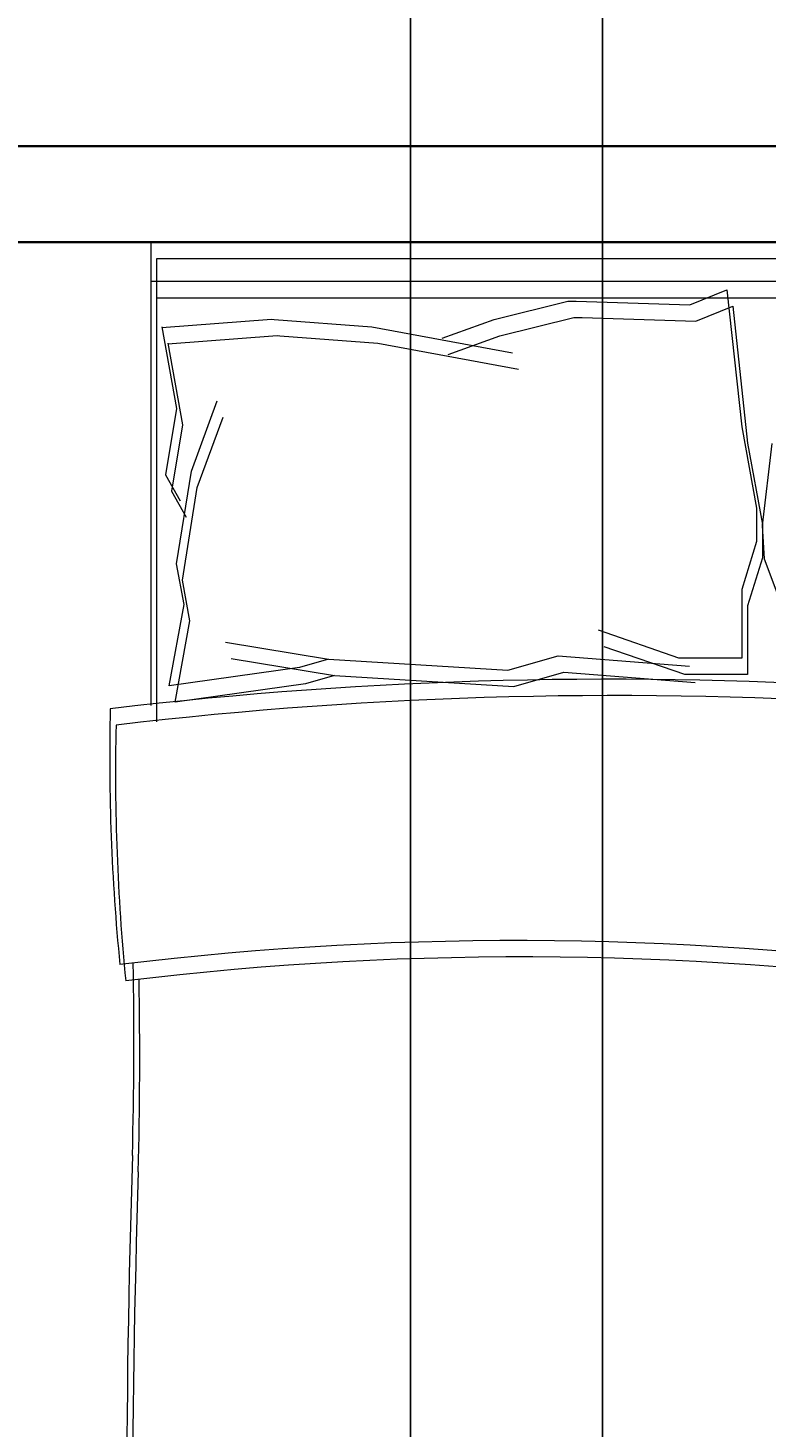
# Model space of a CAD drawing. Units: inches. Extents: x 1088 to 1703, y 668 to 1875.
# Tile 42 of 45: x 1497 to 1531, y 1743 to 1809. Entities that reach past the tile are written whole.
import ezdxf

# ---------------------------------------------------------------- set-up
doc = ezdxf.new("R2010")
doc.units = ezdxf.units.IN
for name, color, linetype, lineweight in [('A-ANNO-DIMS', 2, 'Continuous', 18), ('A-FURN', 8, 'Continuous', 13), ('A-WALL', 7, 'Continuous', 35)]:
    doc.layers.add(name, color=color, linetype=linetype, lineweight=lineweight)
doc.styles.get("Standard").update_dxf_attribs({"font": 'arial.ttf'})
doc.dimstyles.get("Standard").update_dxf_attribs({"dimtxt": 0.18, "dimasz": 0.18, "dimexe": 0.18, "dimexo": 0.0625, "dimgap": 0.09, "dimtad": 0, "dimtih": 1, "dimtoh": 1, "dimdec": 4, "dimzin": 0, "dimdsep": 46, "dimtxsty": 'Standard', "dimcen": 0.09, "dimadec": 0, "dimazin": 0, "dimtfac": 1, "dimtdec": 4, "dimtofl": 0, "dimtmove": 0, "dimatfit": 3, "dimfxl": 1, "dimtolj": 1, "dimtzin": 0, "dimarcsym": 0})

# ---------------------------------------------------------------- blocks, each defined once
blk = doc.blocks.new('BED-DOUBLE')
for p, q in [((0.766, 4.44), (0.766, 61.734)), ((2.605, 4.44), (2.605, 61.734)), ((0, 4.167), (0, 61.46)), ((1.838, 4.167), (1.838, 61.46)), ((14.838, 32.892), (17.044, 33.725)), ((9.422, 32.117), (13.236, 32.81)), ((9.432, 33.249), (13.281, 32.795)), ((13.236, 32.81), (14.796, 32.81)), ((13.281, 32.795), (14.838, 32.892)), ((14.796, 32.81), (17.049, 32.117)), ((8.656, 31.843), (12.469, 32.536)), ((12.469, 32.536), (14.029, 32.536)), ((14.029, 32.536), (16.283, 31.843)), ((2.242, 31.15), (8.656, 31.843)), ((3.008, 31.424), (9.422, 32.117)), ((16.283, 31.843), (19.497, 31.843)), ((17.049, 32.117), (20.264, 32.117)), ((19.497, 31.843), (19.497, 28.897)), ((20.264, 32.117), (20.264, 29.171)), ((2.935, 29.417), (2.242, 31.15)), ((3.702, 29.691), (3.008, 31.424)), ((3.528, 24.361), (3.702, 29.691)), ((20.151, 23.513), (20.635, 29.665)), ((2.762, 24.087), (2.935, 29.417)), ((19.497, 28.897), (18.189, 25.127)), ((20.264, 29.171), (18.956, 25.401)), ((19.384, 23.239), (19.868, 29.391)), ((3.528, 23.975), (3.528, 24.361)), ((2.762, 23.701), (2.762, 24.087)), ((3.629, 20.235), (2.762, 23.701)), ((4.395, 20.509), (3.528, 23.975)), ((20.052, 20.889), (19.384, 23.239)), ((20.819, 21.163), (20.151, 23.513)), ((3.975, 14.516), (5.189, 21.102)), ((4.742, 14.79), (5.955, 21.376)), ((20.302, 12.759), (20.819, 21.163)), ((5.262, 18.083), (4.395, 20.509)), ((19.536, 12.485), (20.052, 20.889)), ((4.495, 17.809), (3.629, 20.235)), ((3.629, 9.933), (3.975, 14.516)), ((4.395, 10.206), (4.742, 14.79)), ((18.736, 7.651), (19.536, 12.485)), ((19.503, 7.925), (20.302, 12.759)), ((19.536, 12.485), (19.923, 11.126)), ((20.302, 12.759), (20.689, 11.4)), ((20.689, 11.4), (21.556, 5.29)), ((19.923, 11.126), (20.789, 5.016)), ((3.607, 9.806), (3.629, 9.933)), ((4.373, 10.08), (4.395, 10.206)), ((4.768, 4.948), (4.373, 10.08)), ((4.002, 4.674), (3.607, 9.806)), ((10.736, 6.056), (7.442, 7.269)), ((11.502, 6.33), (8.209, 7.543)), ((15.069, 5.363), (10.736, 6.056)), ((15.836, 5.637), (11.502, 6.33)), ((17.742, 5.983), (15.836, 5.637)), ((21.556, 5.29), (17.742, 5.983)), ((3.975, 4.67), (7.789, 5.363)), ((4.742, 4.943), (8.555, 5.637)), ((7.789, 5.363), (10.909, 4.843)), ((8.555, 5.637), (11.675, 5.117)), ((10.909, 4.843), (12.122, 5.536)), ((11.675, 5.117), (12.889, 5.81)), ((16.976, 5.709), (15.069, 5.363)), ((20.789, 5.016), (16.976, 5.709)), ((21.712, 4.167), (0, 4.167)), ((22.478, 4.44), (0.766, 4.44))]:
    blk.add_line(p, q)
for centre, radius, start, end in [((187.401, 21.287), 154.676, 171.78449, 186.90062), ((188.167, 21.561), 154.676, 171.78449, 186.90062), ((219.021, 25.88), 197.774, 176.08655, 186.78213), ((218.255, 25.607), 197.774, 176.08655, 186.78213), ((37.373, -200.577), 203.938, 88.4762, 91.00819), ((38.139, -200.304), 203.938, 88.4762, 91.00819), ((60.679, 581.233), 578.221, 268.227709, 271.718541), ((61.445, 581.507), 578.221, 268.227709, 271.718541), ((24.093, 102.097), 99.872, 268.72178, 275.60397), ((24.859, 102.371), 99.872, 268.72178, 275.60397)]:
    blk.add_arc(centre, radius, start, end)
blk = doc.blocks.new('*D28')
at = {"layer": 'A-ANNO-DIMS', "color": 0, "lineweight": -2, "transparency": 16777216}
for p, q in [((1170.345, 1803.621), (1170.345, 1857.788)), ((1170.525, 1857.608), (1408.147, 1857.608)), ((1646.563, 1857.608), (1408.941, 1857.608)), ((1646.743, 1745.552), (1646.743, 1857.788))]:
    blk.add_line(p, q, dxfattribs=at)
at = {"layer": 'A-ANNO-DIMS', "color": 0, "transparency": 16777216}
for points in [[(1170.525, 1857.638), (1170.525, 1857.578), (1170.345, 1857.608)], [(1646.563, 1857.638), (1646.563, 1857.578), (1646.743, 1857.608)]]:
    blk.add_solid(points, dxfattribs=at)
at = {"layer": 'Defpoints', "color": 0, "transparency": 16777216}
for p in [(1646.743, 1857.608), (1170.345, 1803.558), (1646.743, 1745.49)]:
    blk.add_point(p, dxfattribs=at)
at = {"layer": 'A-ANNO-DIMS', "color": 0, "transparency": 16777216, "insert": (1408.544, 1857.608), "char_height": 0.18, "attachment_point": 5}
blk.add_mtext('\\A1;476.4', dxfattribs=at)
blk = doc.blocks.new('*D33')
at = {"layer": 'A-ANNO-DIMS', "color": 0, "lineweight": -2, "transparency": 16777216}
for p, q in [((1514.595, 1355.648), (1514.595, 1857.788)), ((1514.775, 1857.608), (1518.946, 1857.608)), ((1523.415, 1857.608), (1519.244, 1857.608)), ((1523.595, 1331.121), (1523.595, 1857.788))]:
    blk.add_line(p, q, dxfattribs=at)
at = {"layer": 'A-ANNO-DIMS', "color": 0, "transparency": 16777216}
for points in [[(1514.775, 1857.638), (1514.775, 1857.578), (1514.595, 1857.608)], [(1523.415, 1857.638), (1523.415, 1857.578), (1523.595, 1857.608)]]:
    blk.add_solid(points, dxfattribs=at)
at = {"layer": 'Defpoints', "color": 0, "transparency": 16777216}
for p in [(1523.595, 1857.608), (1514.595, 1355.585), (1523.595, 1331.058)]:
    blk.add_point(p, dxfattribs=at)
at = {"layer": 'A-ANNO-DIMS', "color": 0, "transparency": 16777216, "insert": (1519.095, 1857.608), "char_height": 0.18, "attachment_point": 5}
blk.add_mtext('\\A1;9', dxfattribs=at)

msp = doc.modelspace()

# ---------------------------------------------------------------- linework, layer by layer
at = {"layer": 'A-WALL'}
for p, q in [((1437.345, 1803.558), (1624.845, 1803.558)), ((1437.345, 1803.558), (1624.845, 1803.558)), ((1437.345, 1803.558), (1624.845, 1803.558)), ((1437.345, 1803.558), (1624.845, 1803.558)), ((1437.345, 1803.558), (1624.845, 1803.558)), ((1441.845, 1799.058), (1620.345, 1799.058))]:
    msp.add_line(p, q, dxfattribs=at)

# ---------------------------------------------------------------- block references
at = {"layer": 'A-FURN', "rotation": 270}
msp.add_blockref('BED-DOUBLE', (1498.281, 1799.058), dxfattribs=at)

# ---------------------------------------------------------------- dimensions: what is measured, and where the dimension line sits
at = {"layer": 'A-ANNO-DIMS'}
for base, p1, p2, override, picture, middle in [((1646.743, 1857.608), (1170.345, 1803.558), (1646.743, 1745.49), {"dimdec": 1, "dimlfac": 1, "dimrnd": 0, "dimzin": 0, "dimdsep": 46, "dimlunit": 2}, '*D28', (1408.544, 1857.608)), ((1523.595, 1857.608), (1514.595, 1355.585), (1523.595, 1331.058), {"dimdec": 0, "dimlfac": 1, "dimrnd": 0, "dimzin": 0, "dimdsep": 46, "dimlunit": 2}, '*D33', (1519.095, 1857.608))]:
    dim = msp.add_linear_dim(base=base, p1=p1, p2=p2, dimstyle='Standard', override=override, dxfattribs=at)
    dim.commit()
    dim.dimension.update_dxf_attribs({"geometry": picture, "text_midpoint": middle})

doc.saveas('drawing.dxf')
